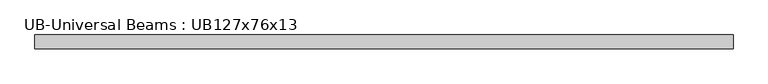
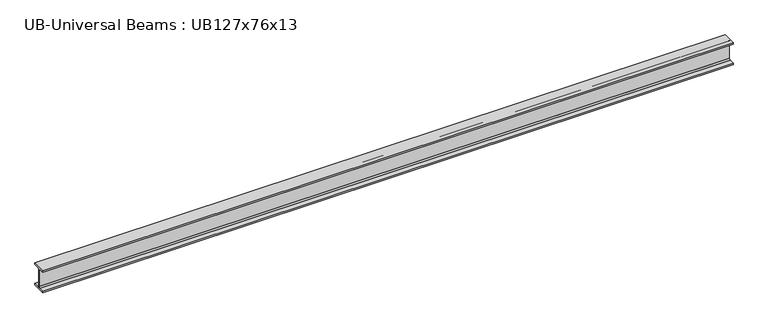
"""IFC4 building model written with IfcOpenShell, lengths in millimetres: member geometry, UB-Universal Beams : UB127x76x13."""

from ifc_helpers import new_model, si_unit, point, frame, frame_2d, origin, place, context, project, spatial, polyline, circle_curve, trimmed, segment, composite_curve, outline, extrude, source, transform, mapped, element, save


def ub_universal_beams_ub127x76x13_5fda7735(model_context):
    return source(origin(), model_context, "Body", "SweptSolid", [
        extrude(outline(composite_curve([segment(polyline([(38.0, -55.9), (38.0, -63.5), (-38.0, -63.5), (-38.0, -55.9), (-9.6, -55.9)]), True, "CONTINUOUS"), segment(trimmed(circle_curve(frame_2d((-9.6, -48.3)), 7.6), [point((-9.6, -55.9))], [point((-2.0, -48.3))], True, "CARTESIAN"), True, "CONTINUOUS"), segment(polyline([(-2.0, -48.3), (-2.0, 48.3)]), True, "CONTINUOUS"), segment(trimmed(circle_curve(frame_2d((-9.6, 48.3)), 7.6), [point((-2.0, 48.3))], [point((-9.6, 55.9))], True, "CARTESIAN"), True, "CONTINUOUS"), segment(polyline([(-9.6, 55.9), (-38.0, 55.9), (-38.0, 63.5), (38.0, 63.5), (38.0, 55.9), (9.6, 55.9)]), True, "CONTINUOUS"), segment(trimmed(circle_curve(frame_2d((9.6, 48.3)), 7.6), [point((9.6, 55.9))], [point((2.0, 48.3))], True, "CARTESIAN"), True, "CONTINUOUS"), segment(polyline([(2.0, 48.3), (2.0, -48.3)]), True, "CONTINUOUS"), segment(trimmed(circle_curve(frame_2d((9.6, -48.3)), 7.6), [point((2.0, -48.3))], [point((9.6, -55.9))], True, "CARTESIAN"), True, "CONTINUOUS"), segment(polyline([(9.6, -55.9), (38.0, -55.9)]), True, "CONTINUOUS")], self_intersect=False)), frame((-2128.0, 0.0, 0.0), z_axis=(1.0, 0.0, 0.0), x_axis=(0.0, 1.0, 0.0)), (0.0, 0.0, 1.0), 3816.1),
    ])


if __name__ == "__main__":
    model = new_model("IFC4")
    model_context = context("Model", 3, world=origin())
    ifc_project = project(units=[si_unit("LENGTHUNIT", "METRE", prefix="MILLI")], contexts=[model_context])
    site = spatial("IfcSite", under=ifc_project)
    building = spatial("IfcBuilding", under=site)
    placement = place(None, origin())
    ub_universal_beams_ub127x76x13_shape = ub_universal_beams_ub127x76x13_5fda7735(model_context)
    element("IfcMember", 1, ObjectType="UB-Universal Beams : UB127x76x13", at=placement, inside=building, context=model_context, shape_type="MappedRepresentation", body=[
        mapped(ub_universal_beams_ub127x76x13_shape, transform((0.0, 0.0, 0.0), x_axis=(1.0, 0.0, 0.0), y_axis=(0.0, 1.0, 0.0), z_axis=(0.0, 0.0, 1.0))),
    ])
    save(model, "model.ifc")

# Revit data of these elements
# Type "UB-Universal Beams : UB127x76x13"
#   Section Name Key = "UB127X76X13"
#   Width = 7.6 cm
#   Web Thickness = 0.4 cm
#   Web Fillet = 0.76 cm
#   Warping Constant = 2000.0 cm⁶
#   Torsional Moment of Inertia = 2.85 cm⁴
#   Section Area = 16.5 cm²
#   Plastic Modulus weak axis = 22.6 cm³
#   Plastic Modulus strong axis = 84.2 cm³
#   Nominal Weight = 13.00 kgf/m
#   Moment of Inertia weak axis = 55.70 cm⁴
#   Moment of Inertia strong axis = 473.00 cm⁴
#   Height = 12.7 cm
#   Flange Thickness = 0.76 cm
#   Elastic Modulus weak axis = 14.7 cm³
#   Elastic Modulus strong axis = 74.6 cm³
#   Centroid Vertical = 6.35 cm
#   Centroid Horizontal = 3.8 cm
#   Bolt Spacing = 4.0 cm
#   Length [instance default] = 1.5 m
#   Structural Material [instance default] = Metal - Steel 43-275
#   Type Comments = ""
#   Assembly Code = ""
# Element 1 (IfcMember, "UB-Universal Beams : UB127x76x13")
#   Materials on its faces: "Metal - Steel 43-275"
# Materials
#   "Metal - Steel 43-275": class "Metal", colour RGB 247 247 247, transparency 0, Cost = 0
